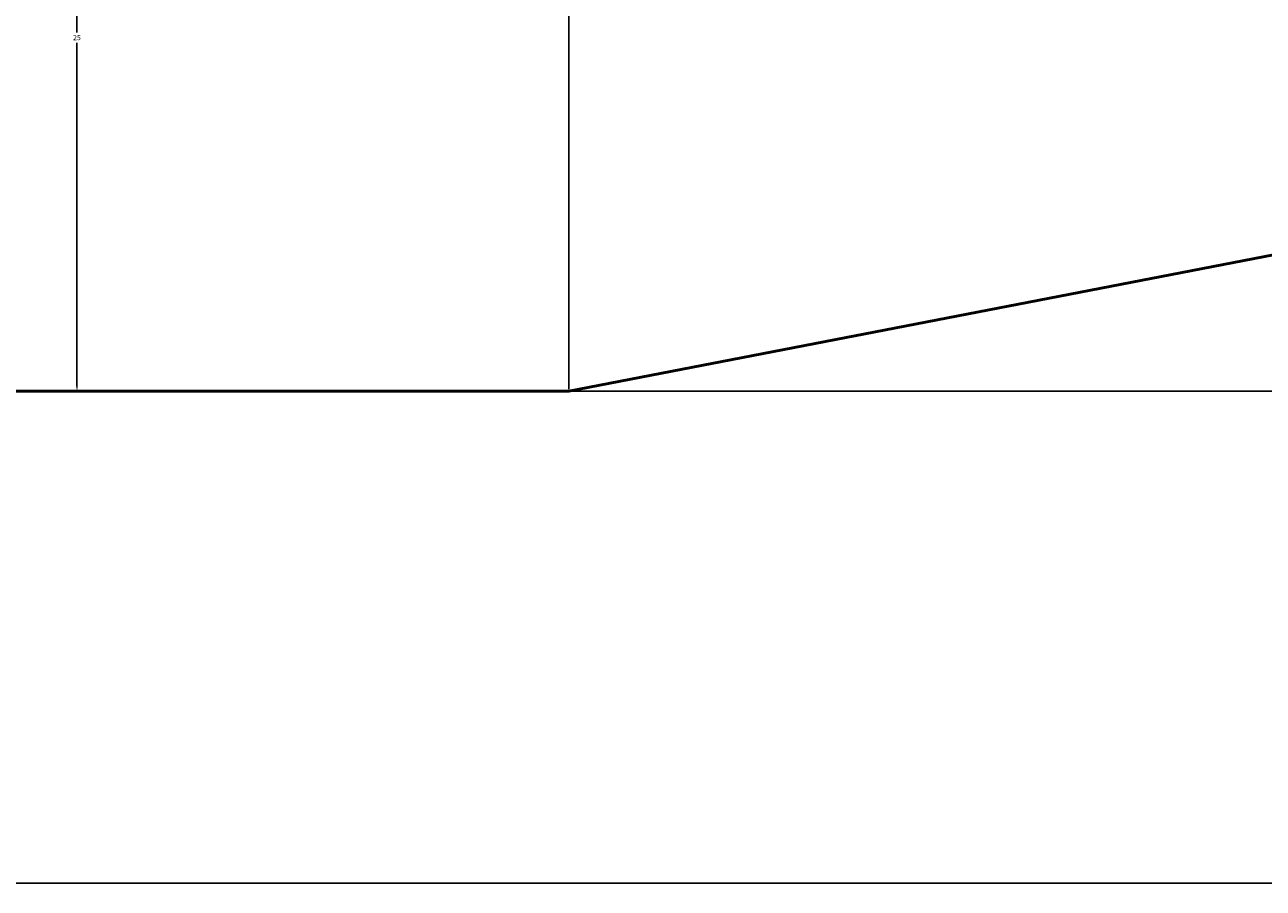
# Model space of a CAD drawing. Units: inches. Extents: x 457 to 775, y 319 to 541.
# Tile 2 of 12: x 536 to 580, y 319 to 350. Entities that reach past the tile are written whole.
import ezdxf

# ---------------------------------------------------------------- set-up
doc = ezdxf.new("R2010")
doc.units = ezdxf.units.IN
doc.header["$MEASUREMENT"] = 0
doc.layers.add('M-DIMS', color=2, linetype='Continuous', lineweight=18)
doc.layers.add('M-OUTL', color=7, linetype='Continuous', lineweight=50)
doc.styles.get("Standard").update_dxf_attribs({"font": 'arial.ttf'})
doc.dimstyles.get("Standard").update_dxf_attribs({"dimtxt": 0.18, "dimasz": 0.18, "dimexe": 0.18, "dimexo": 0.0625, "dimgap": 0.09, "dimtad": 0, "dimtih": 1, "dimtoh": 1, "dimdec": 4, "dimzin": 0, "dimdsep": 46, "dimtxsty": 'Standard', "dimcen": 0.09, "dimadec": 0, "dimazin": 0, "dimtfac": 1, "dimtdec": 4, "dimtofl": 0, "dimtmove": 0, "dimatfit": 3, "dimfxl": 1, "dimtolj": 1, "dimtzin": 0, "dimarcsym": 0})

# ---------------------------------------------------------------- blocks, each defined once
blk = doc.blocks.new('*D2')
at = {"layer": 'Defpoints', "color": 0, "transparency": 16777216}
for p in [(756.931, 375.696), (474.306, 336.696), (756.931, 319.296)]:
    blk.add_point(p, dxfattribs=at)
at = {"layer": 'M-DIMS', "color": 0, "lineweight": -2, "transparency": 16777216}
for p, q in [((756.931, 375.634), (756.931, 319.116)), ((474.306, 336.634), (474.306, 319.116)), ((474.486, 319.296), (615.223, 319.296)), ((756.751, 319.296), (616.014, 319.296))]:
    blk.add_line(p, q, dxfattribs=at)
at = {"layer": 'M-DIMS', "color": 0, "transparency": 16777216}
for points in [[(474.486, 319.326), (474.486, 319.266), (474.306, 319.296)], [(756.751, 319.326), (756.751, 319.266), (756.931, 319.296)]]:
    blk.add_solid(points, dxfattribs=at)
at = {"layer": 'M-DIMS', "color": 0, "transparency": 16777216, "insert": (615.619, 319.296), "char_height": 0.18, "attachment_point": 5}
blk.add_mtext('\\A1;282.6', dxfattribs=at)
blk = doc.blocks.new('*D3')
at = {"layer": 'Defpoints', "color": 0, "transparency": 16777216}
for p in [(456.906, 523.213), (646.001, 523.213), (474.306, 336.696)]:
    blk.add_point(p, dxfattribs=at)
at = {"layer": 'M-DIMS', "color": 0, "lineweight": -2, "transparency": 16777216}
for p, q in [((645.939, 523.213), (456.726, 523.213)), ((456.906, 523.033), (456.906, 430.136)), ((456.906, 336.876), (456.906, 429.773)), ((474.244, 336.696), (456.726, 336.696))]:
    blk.add_line(p, q, dxfattribs=at)
at = {"layer": 'M-DIMS', "color": 0, "transparency": 16777216}
for points in [[(456.876, 523.033), (456.936, 523.033), (456.906, 523.213)], [(456.876, 336.876), (456.936, 336.876), (456.906, 336.696)]]:
    blk.add_solid(points, dxfattribs=at)
at = {"layer": 'M-DIMS', "color": 0, "transparency": 16777216, "insert": (456.906, 429.954), "char_height": 0.18, "attachment_point": 5}
blk.add_mtext('\\A1;186.5', dxfattribs=at)
blk = doc.blocks.new('*D6')
at = {"layer": 'Defpoints', "color": 0, "transparency": 16777216}
for p in [(554.931, 354.096), (474.306, 336.696), (554.931, 336.696)]:
    blk.add_point(p, dxfattribs=at)
at = {"layer": 'M-DIMS', "color": 0, "lineweight": -2, "transparency": 16777216}
for p, q in [((474.306, 336.759), (474.306, 354.276)), ((554.931, 336.759), (554.931, 354.276)), ((474.486, 354.096), (514.226, 354.096)), ((554.751, 354.096), (515.011, 354.096))]:
    blk.add_line(p, q, dxfattribs=at)
at = {"layer": 'M-DIMS', "color": 0, "transparency": 16777216}
for points in [[(474.486, 354.126), (474.486, 354.066), (474.306, 354.096)], [(554.751, 354.126), (554.751, 354.066), (554.931, 354.096)]]:
    blk.add_solid(points, dxfattribs=at)
at = {"layer": 'M-DIMS', "color": 0, "transparency": 16777216, "insert": (514.619, 354.096), "char_height": 0.18, "attachment_point": 5}
blk.add_mtext('\\A1;80.62', dxfattribs=at)
blk = doc.blocks.new('*D7')
at = {"layer": 'Defpoints', "color": 0, "transparency": 16777216}
for p in [(537.531, 361.696), (554.931, 361.696), (554.931, 336.696)]:
    blk.add_point(p, dxfattribs=at)
at = {"layer": 'M-DIMS', "color": 0, "lineweight": -2, "transparency": 16777216}
for p, q in [((554.869, 361.696), (537.351, 361.696)), ((537.531, 361.516), (537.531, 349.378)), ((537.531, 336.876), (537.531, 349.014)), ((554.869, 336.696), (537.351, 336.696))]:
    blk.add_line(p, q, dxfattribs=at)
at = {"layer": 'M-DIMS', "color": 0, "transparency": 16777216}
for points in [[(537.501, 361.516), (537.561, 361.516), (537.531, 361.696)], [(537.501, 336.876), (537.561, 336.876), (537.531, 336.696)]]:
    blk.add_solid(points, dxfattribs=at)
at = {"layer": 'M-DIMS', "color": 0, "transparency": 16777216, "insert": (537.531, 349.196), "char_height": 0.18, "attachment_point": 5}
blk.add_mtext('\\A1;25', dxfattribs=at)
blk = doc.blocks.new('*D9')
at = {"layer": 'Defpoints', "color": 0, "transparency": 16777216}
for p in [(756.931, 375.696), (774.331, 375.696), (554.931, 336.696)]:
    blk.add_point(p, dxfattribs=at)
at = {"layer": 'M-DIMS', "color": 0, "lineweight": -2, "transparency": 16777216}
for p, q in [((756.994, 375.696), (774.511, 375.696)), ((774.331, 375.516), (774.331, 356.378)), ((774.331, 336.876), (774.331, 356.014)), ((554.994, 336.696), (774.511, 336.696))]:
    blk.add_line(p, q, dxfattribs=at)
at = {"layer": 'M-DIMS', "color": 0, "transparency": 16777216}
for points in [[(774.301, 375.516), (774.361, 375.516), (774.331, 375.696)], [(774.301, 336.876), (774.361, 336.876), (774.331, 336.696)]]:
    blk.add_solid(points, dxfattribs=at)
at = {"layer": 'M-DIMS', "color": 0, "transparency": 16777216, "insert": (774.331, 356.196), "char_height": 0.18, "attachment_point": 5}
blk.add_mtext('\\A1;39', dxfattribs=at)

msp = doc.modelspace()

# ---------------------------------------------------------------- linework, layer by layer
at = {"layer": 'M-OUTL'}
for q in [(756.931, 375.696), (474.306, 336.696)]:
    msp.add_line((554.931, 336.696), q, dxfattribs=at)

# ---------------------------------------------------------------- dimensions: what is measured, and where the dimension line sits
at = {"layer": 'M-DIMS'}
for base, p1, p2, override, picture, middle in [((456.906, 523.213), (474.306, 336.696), (646.001, 523.213), {"dimdec": 1, "dimlfac": 1, "dimrnd": 0, "dimzin": 0, "dimdsep": 46, "dimlunit": 2}, '*D3', (456.906, 429.954)), ((774.331, 375.696), (554.931, 336.696), (756.931, 375.696), {"dimdec": 0, "dimlfac": 1, "dimrnd": 0, "dimzin": 0, "dimdsep": 46, "dimlunit": 2}, '*D9', (774.331, 356.196)), ((537.531, 361.696), (554.931, 336.696), (554.931, 361.696), {"dimdec": 0, "dimlfac": 1, "dimrnd": 0, "dimzin": 0, "dimdsep": 46, "dimlunit": 2}, '*D7', (537.531, 349.196))]:
    dim = msp.add_linear_dim(base=base, p1=p1, p2=p2, angle=90, dimstyle='Standard', override=override, dxfattribs=at)
    dim.commit()
    dim.dimension.update_dxf_attribs({"geometry": picture, "text_midpoint": middle})
for base, p1, p2, override, picture, middle in [((756.931, 319.296), (474.306, 336.696), (756.931, 375.696), {"dimdec": 1, "dimlfac": 1, "dimrnd": 0, "dimzin": 0, "dimdsep": 46, "dimlunit": 2}, '*D2', (615.619, 319.296)), ((554.931, 354.096), (474.3061, 336.696), (554.931, 336.696), {"dimdec": 2, "dimlfac": 1, "dimrnd": 0, "dimzin": 0, "dimdsep": 46, "dimlunit": 2}, '*D6', (514.6186, 354.096))]:
    dim = msp.add_linear_dim(base=base, p1=p1, p2=p2, dimstyle='Standard', override=override, dxfattribs=at)
    dim.commit()
    dim.dimension.update_dxf_attribs({"geometry": picture, "text_midpoint": middle})

doc.saveas('drawing.dxf')
